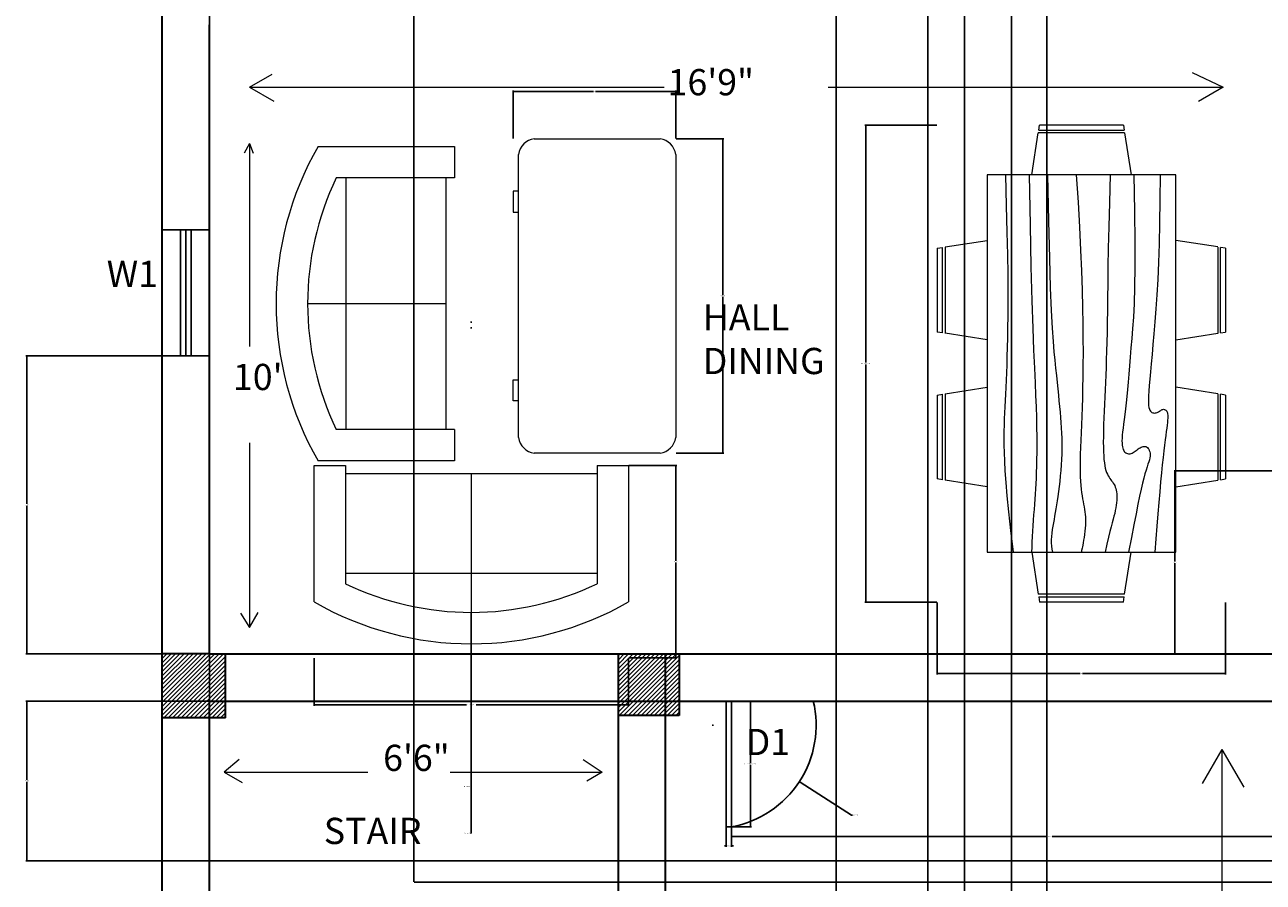
# Model space of a CAD drawing. Units: inches. Extents: x -4 to 429, y -457 to 84.
# Tile 2 of 4: x -4 to 232, y -295 to -131. Entities that reach past the tile are written whole.
import ezdxf

# ---------------------------------------------------------------- set-up
doc = ezdxf.new("R2010")
doc.units = ezdxf.units.IN
doc.header["$MEASUREMENT"] = 0
for name, color, linetype, lineweight in [('A-ANNO-DIMS', 2, 'Continuous', 18), ('A-ANNO-TEXT', 3, 'Continuous', 18), ('A-AREA-IDEN', 7, 'Continuous', 25), ('A-COLS', 7, 'Continuous', 35), ('A-COLS-PATT', 252, 'Continuous', 13), ('A-DOOR', 3, 'Continuous', 25), ('A-FURN', 8, 'Continuous', 18), ('A-GLAZ', 4, 'Continuous', 25), ('A-WALL', 7, 'Continuous', 35)]:
    doc.layers.add(name, color=color, linetype=linetype, lineweight=lineweight)
doc.styles.get("Standard").update_dxf_attribs({"font": 'arial.ttf'})
doc.dimstyles.get("Standard").update_dxf_attribs({"dimtxt": 0.18, "dimasz": 0.18, "dimexe": 0.18, "dimexo": 0.0625, "dimgap": 0.09, "dimtad": 0, "dimtih": 1, "dimtoh": 1, "dimdec": 4, "dimzin": 0, "dimdsep": 46, "dimtxsty": 'Standard', "dimcen": 0.09, "dimadec": 0, "dimazin": 0, "dimtfac": 1, "dimtdec": 4, "dimtofl": 0, "dimtmove": 0, "dimatfit": 3, "dimfxl": 1, "dimtolj": 1, "dimtzin": 0, "dimarcsym": 0})
pattern_1 = [(45, (-1330.13025, -719.5531), (-0.41542523, 0.41542523), [])]

# ---------------------------------------------------------------- blocks, each defined once
blk = doc.blocks.new('Dining Set - 36 x 72 in.')
for p, q in [((-22.2343, 26.00059), (-23.4847, 17.99762)), ((-22.2304, 26), (-5.7608, 26)), ((-22, 27.5), (-22.1562, 26.50042)), ((-5.8416, 26.5), (-22.1534, 26.5)), ((-22, 27.5), (-6, 27.5)), ((-5.8437, 26.49966), (-6, 27.5)), ((-4.5152, 17.99762), (-5.7655, 25.99926)), ((5.7657, 26.00059), (4.5153, 17.99762)), ((5.7696, 26), (22.2392, 26)), ((6, 27.5), (5.8438, 26.50042)), ((22.1584, 26.5), (5.8466, 26.5)), ((6, 27.5), (22, 27.5)), ((22.1563, 26.49966), (22, 27.5)), ((23.4848, 17.99762), (22.2345, 25.99926)), ((36, 18), (-36, 18)), ((-36, 18), (-36, -18)), ((36, -18), (36, 18)), ((-44.0006, 8.23428), (-35.9976, 9.48474)), ((44.0006, 8.23428), (35.9976, 9.48474)), ((-45.5, 8), (-44.5004, 8.15617)), ((-45.5, 8), (-45.5, -8)), ((-44.5, -8.15843), (-44.5, 8.15338)), ((-44, 8.23041), (-44, -8.23915)), ((44, 8.23041), (44, -8.23915)), ((44.5, -8.15843), (44.5, 8.15338)), ((45.5, 8), (44.5005, 8.15617)), ((45.5, 8), (45.5, -8)), ((-44.4997, -8.15631), (-45.5, -8)), ((-35.9976, -9.48476), (-43.9993, -8.2345)), ((35.9976, -9.48476), (43.9993, -8.2345)), ((44.4997, -8.15631), (45.5, -8)), ((-36, -18), (36, -18)), ((-22.2343, -26.0006), (-23.4847, -17.99762)), ((-4.5152, -17.99762), (-5.7655, -25.99928)), ((5.7657, -26.0006), (4.5153, -17.99762)), ((23.4848, -17.99762), (22.2345, -25.99928)), ((-22.2304, -26), (-5.7608, -26)), ((-22, -27.5), (-22.1562, -26.50044)), ((-5.8416, -26.5), (-22.1534, -26.5)), ((-22, -27.5), (-6, -27.5)), ((-5.8437, -26.49967), (-6, -27.5)), ((5.7696, -26), (22.2392, -26)), ((6, -27.5), (5.8438, -26.50044)), ((22.1584, -26.5), (5.8466, -26.5)), ((6, -27.5), (22, -27.5)), ((22.1563, -26.49967), (22, -27.5))]:
    blk.add_line(p, q)
for points in [[(-36, 15), (-31.1772, 14.97754), (-26.8079, 14.91406), (-22.8538, 14.81543), (-19.276, 14.6875), (-16.0362, 14.53613), (-13.0957, 14.36718), (-10.4159, 14.18652), (-7.9583, 14), (-5.6904, 13.81315), (-3.6035, 13.63021), (-1.6954, 13.45508), (0.0365, 13.29166), (1.5945, 13.14388), (2.9811, 13.01562), (4.1988, 12.9108), (5.25, 12.83333), (6.1393, 12.78613), (6.8802, 12.76823), (7.4883, 12.77767), (7.9792, 12.8125), (8.3685, 12.87077), (8.6719, 12.95052), (8.9049, 13.0498), (9.0833, 13.16666), (9.2205, 13.29899), (9.3216, 13.44401), (9.3895, 13.59879), (9.4271, 13.76041), (9.4373, 13.92594), (9.4232, 14.09245), (9.3875, 14.257), (9.3333, 14.41666), (9.2638, 14.56917), (9.1836, 14.71484), (9.0975, 14.85465), (9.0104, 14.98958), (8.9272, 15.1206), (8.8529, 15.2487), (8.7922, 15.37483), (8.75, 15.5), (8.7305, 15.62467), (8.7344, 15.74739), (8.7617, 15.86621), (8.8125, 15.97916), (8.8867, 16.08431), (8.9844, 16.17968), (9.1055, 16.26334), (9.25, 16.33333), (9.4189, 16.38802), (9.6172, 16.42708), (9.8506, 16.45052), (10.125, 16.45833), (10.4463, 16.45052), (10.8203, 16.42708), (11.2529, 16.38802), (11.75, 16.33333), (12.3184, 16.26318), (12.9694, 16.17838), (13.7151, 16.07991), (14.5677, 15.96875), (15.5395, 15.84586), (16.6426, 15.71224), (17.8893, 15.56884), (19.2917, 15.41666), (20.859, 15.25667), (22.5879, 15.08984), (24.4721, 14.91715), (26.5052, 14.73958), (28.6809, 14.5581), (30.9929, 14.3737), (33.4347, 14.18733), (36, 14)], [(-36, 10), (-28.9766, 10.14274), (-23.1725, 10.20442), (-18.4241, 10.19775), (-14.5677, 10.13541), (-11.4399, 10.03011), (-8.877, 9.89453), (-6.7154, 9.74137), (-4.7917, 9.58333), (-2.9698, 9.43082), (-1.2246, 9.28515), (0.4415, 9.14534), (2.026, 9.01041), (3.5266, 8.87939), (4.9408, 8.7513), (6.266, 8.62516), (7.5, 8.5), (8.6411, 8.37549), (9.6914, 8.2539), (10.6538, 8.13818), (11.5312, 8.03125), (12.3267, 7.93603), (13.043, 7.85547), (13.6831, 7.79248), (14.25, 7.75), (14.7471, 7.7303), (15.1797, 7.73307), (15.5537, 7.75732), (15.875, 7.80208), (16.1494, 7.86637), (16.3828, 7.94922), (16.5811, 8.04964), (16.75, 8.16666), (16.8944, 8.29915), (17.0143, 8.44531), (17.1089, 8.60319), (17.1771, 8.77083), (17.218, 8.94629), (17.2305, 9.1276), (17.2137, 9.31282), (17.1667, 9.5), (17.0895, 9.6875), (16.987, 9.875), (16.8649, 10.0625), (16.7292, 10.25), (16.5856, 10.4375), (16.4401, 10.625), (16.2985, 10.8125), (16.1667, 11), (16.05, 11.18733), (15.9518, 11.3737), (15.8752, 11.5581), (15.8229, 11.73958), (15.798, 11.91715), (15.8034, 12.08984), (15.842, 12.25667), (15.9167, 12.41666), (16.0295, 12.56836), (16.1784, 12.70833), (16.3605, 12.83268), (16.5729, 12.9375), (16.8127, 13.01888), (17.0768, 13.07291), (17.3625, 13.0957), (17.6667, 13.08333), (17.9894, 13.03312), (18.3418, 12.94726), (18.7382, 12.82918), (19.1927, 12.68229), (19.7195, 12.51001), (20.3327, 12.31575), (21.0465, 12.10294), (21.875, 11.875), (22.8357, 11.63354), (23.959, 11.37304), (25.2786, 11.08618), (26.8282, 10.76562), (28.6414, 10.40405), (30.752, 9.99414), (33.1936, 9.52856), (36, 9)], [(-36, 5.5), (-30.7157, 5.3348), (-26.069, 5.20963), (-21.9946, 5.11767), (-18.4271, 5.05208), (-15.3009, 5.00602), (-12.5508, 4.97265), (-10.1112, 4.94515), (-7.9167, 4.91666), (-5.909, 4.88167), (-4.0586, 4.83984), (-2.3429, 4.79215), (-0.7396, 4.73958), (0.7739, 4.6831), (2.22, 4.6237), (3.6213, 4.56233), (5, 4.5), (6.373, 4.43782), (7.7344, 4.3776), (9.0723, 4.32129), (10.375, 4.27083), (11.6309, 4.22819), (12.8281, 4.19531), (13.9551, 4.17415), (15, 4.16666), (15.954, 4.17448), (16.819, 4.19791), (17.6001, 4.23698), (18.3021, 4.29166), (18.9299, 4.36198), (19.4883, 4.44791), (19.9823, 4.54948), (20.4167, 4.66666), (20.7969, 4.79899), (21.1302, 4.94401), (21.4245, 5.09879), (21.6875, 5.26041), (21.9271, 5.42594), (22.1511, 5.59245), (22.3672, 5.757), (22.5834, 5.91666), (22.8065, 6.06868), (23.0404, 6.21093), (23.2879, 6.34147), (23.5521, 6.45833), (23.8358, 6.55957), (24.142, 6.64323), (24.4735, 6.70735), (24.8334, 6.75), (25.2235, 6.76969), (25.642, 6.76692), (26.0858, 6.74267), (26.5521, 6.69791), (27.0379, 6.63362), (27.5404, 6.55078), (28.0565, 6.45036), (28.5834, 6.33333), (29.1242, 6.19987), (29.7071, 6.04687), (30.3661, 5.87044), (31.1354, 5.66666), (32.0493, 5.43164), (33.142, 5.16146), (34.4475, 4.85221), (36, 4.5)], [(-36, -1), (-30.7915, -0.6591), (-26.0195, -0.38216), (-21.6519, -0.16284), (-17.6563, 0.00521), (-14.0005, 0.12833), (-10.6523, 0.21289), (-7.5796, 0.26522), (-4.75, 0.29166), (-2.134, 0.29793), (0.2878, 0.28711), (2.5317, 0.26163), (4.6146, 0.22396), (6.5529, 0.17651), (8.3633, 0.12174), (10.0623, 0.06209), (11.6667, 0), (13.1899, -0.06201), (14.6341, -0.1211), (15.9982, -0.17432), (17.2813, -0.21875), (18.4823, -0.25147), (19.6003, -0.26953), (20.6343, -0.27002), (21.5834, -0.25), (22.4481, -0.20768), (23.2357, -0.14584), (23.9549, -0.06836), (24.6146, 0.02083), (25.2235, 0.11784), (25.7904, 0.21875), (26.3241, 0.31966), (26.8334, 0.41666), (27.3265, 0.50618), (27.8099, 0.58593), (28.2894, 0.65397), (28.7709, 0.70833), (29.2601, 0.74707), (29.763, 0.76823), (30.2855, 0.76985), (30.8334, 0.75), (31.4088, 0.70784), (31.9994, 0.64713), (32.589, 0.57275), (33.1615, 0.48958), (33.7008, 0.4025), (34.1908, 0.3164), (34.6153, 0.23616), (34.9584, 0.16666), (35.2099, 0.11165), (35.3848, 0.07031), (35.504, 0.04069), (35.5886, 0.02083), (35.6594, 0.00879), (35.7377, 0.0026), (35.8442, 0.00032), (36, 0)], [(-36, -6.5), (-27.1843, -6.31267), (-20.084, -6.1263), (-14.469, -5.9419), (-10.1094, -5.76042), (-6.7752, -5.58285), (-4.2363, -5.41016), (-2.2629, -5.24333), (-0.625, -5.08334), (0.8708, -4.93099), (2.2715, -4.78646), (3.5872, -4.64974), (4.8281, -4.52084), (6.0046, -4.39974), (7.127, -4.28646), (8.2053, -4.18099), (9.25, -4.08334), (10.2705, -3.99382), (11.2734, -3.91407), (12.2647, -3.84603), (13.25, -3.79167), (14.2354, -3.75293), (15.2266, -3.73177), (16.2295, -3.73015), (17.25, -3.75), (18.2912, -3.79248), (19.3451, -3.85547), (20.4009, -3.93604), (21.4479, -4.03125), (22.4754, -4.13819), (23.4727, -4.25391), (24.4289, -4.37549), (25.3334, -4.5), (26.1785, -4.62492), (26.9694, -4.74935), (27.7145, -4.87281), (28.4219, -4.99479), (29.1, -5.11483), (29.7572, -5.23242), (30.4016, -5.34709), (31.0417, -5.45834), (31.6837, -5.56437), (32.3262, -5.65821), (32.9658, -5.73153), (33.599, -5.77604), (34.2224, -5.78345), (34.8327, -5.74545), (35.4264, -5.65373), (36, -5.5)], [(-36, -10), (-26.4022, -9.81299), (-18.4675, -9.62891), (-11.9839, -9.45069), (-6.7396, -9.28125), (-2.5226, -9.12354), (0.8789, -8.98047), (3.6769, -8.85498), (6.0833, -8.75), (8.2767, -8.66765), (10.3021, -8.60677), (12.1712, -8.56543), (13.8958, -8.54167), (15.4876, -8.53353), (16.9583, -8.53907), (18.3197, -8.55632), (19.5834, -8.58334), (20.7616, -8.61841), (21.8685, -8.66081), (22.9188, -8.71004), (23.9271, -8.76563), (24.9081, -8.82707), (25.8763, -8.89388), (26.8465, -8.96558), (27.8334, -9.04167), (28.8474, -9.12118), (29.8828, -9.20117), (30.93, -9.27824), (31.9792, -9.34896), (33.0205, -9.40991), (34.0443, -9.45768), (35.0407, -9.48885), (36, -9.5)], [(-36, -14.5), (-30.0881, -14.33513), (-25.0332, -14.21224), (-20.7312, -14.12647), (-17.0781, -14.07292), (-13.97, -14.04671), (-11.3027, -14.04297), (-8.9724, -14.05681), (-6.875, -14.08334), (-4.9224, -14.11833), (-3.0905, -14.16016), (-1.3709, -14.20785), (0.2448, -14.26042), (1.7647, -14.3169), (3.1973, -14.3763), (4.5507, -14.43767), (5.8333, -14.5), (7.0554, -14.5621), (8.235, -14.62175), (9.3922, -14.67652), (10.5469, -14.72396), (11.7192, -14.76164), (12.929, -14.78711), (14.1965, -14.79794), (15.5417, -14.79167), (16.9933, -14.76424), (18.6152, -14.70508), (20.4804, -14.60197), (22.6615, -14.44271), (25.2312, -14.21509), (28.2624, -13.9069), (31.8277, -13.50594), (36, -13)]]:
    blk.add_lwpolyline(points)
blk = doc.blocks.new('Sofa - Roundback Loveseat 5 ft.')
for p, q in [((0, -32.44198), (0, -5.99998)), ((-24, -33.99998), (-24, -11.46958)), ((24.00004, -33.99998), (24.00004, -11.46958)), ((-23.9998, -13.38178), (23.99986, -13.38178)), ((-24, -32.44198), (24.00004, -32.44198))]:
    blk.add_line(p, q)
for points in [[(-24, -33.99998), (-30, -33.99998), (-30, -7.99998)], [(30.00004, -7.99998), (30.00004, -33.99998), (24.00004, -33.99998)]]:
    blk.add_lwpolyline(points)
for centre, radius, start, end in [((0, -60.24998), 60.24998, 60.13715, 119.8628), ((0, -61.38438), 55.38444, 64.32083, 115.6792)]:
    blk.add_arc(centre, radius, start, end)
blk = doc.blocks.new('Desk - 30 x 60 in.')
for p, q in [((-26.999995, 0), (26.999995, 0)), ((-29.999995, -27), (-29.999995, -3)), ((29.999995, -3), (29.999995, -27)), ((26.999995, -30), (-26.999995, -30)), ((-20.000005, -30), (-20.000005, -31)), ((-16.000005, -31), (-16.000005, -30)), ((15.999995, -31), (15.999995, -30)), ((19.999995, -30), (19.999995, -31)), ((-20.000005, -31), (-16.000005, -31)), ((19.999995, -31), (15.999995, -31))]:
    blk.add_line(p, q)
for centre, start, end in [((-26.499995, -3.5), 98.1301, 171.8699), ((26.499995, -3.5), 8.130102, 81.8699), ((-26.499995, -26.5), 188.1301, 261.8699), ((26.499995, -26.5), 278.1301, 351.8699)]:
    blk.add_arc(centre, 3.535534, start, end)
blk = doc.blocks.new('WIN-24IN-9IN-WALL')
for p, q in [((0, 5.5), (24, 5.5)), ((0, 4.5), (24, 4.5)), ((0, 3.5), (24, 3.5))]:
    blk.add_line(p, q)
blk.add_lwpolyline([(0, 9), (24, 9), (24, 0), (0, 0)], close=True)
blk = doc.blocks.new('DOOR-LEAF-24IN')
for p, q in [((0, 0), (0, 24)), ((0, 24), (1, 24)), ((1, 24), (1, 0))]:
    blk.add_line(p, q)
blk = doc.blocks.new('*D14')
at = {"layer": 'A-ANNO-DIMS', "color": 0, "lineweight": -2, "transparency": 16777216}
for p, q in [((130.7, -260.34), (134.41, -260.34)), ((134.23, -260.52), (134.23, -272.16)), ((134.23, -284.16), (134.23, -272.52)), ((130.7, -284.34), (134.41, -284.34))]:
    blk.add_line(p, q, dxfattribs=at)
at = {"layer": 'A-ANNO-DIMS', "color": 0, "transparency": 16777216}
for points in [[(134.2, -260.52), (134.26, -260.52), (134.23, -260.34)], [(134.2, -284.16), (134.26, -284.16), (134.23, -284.34)]]:
    blk.add_solid(points, dxfattribs=at)
at = {"layer": 'Defpoints', "color": 0, "transparency": 16777216}
for p in [(130.63, -260.34), (130.63, -284.34), (134.23, -284.34)]:
    blk.add_point(p, dxfattribs=at)
at = {"layer": 'A-ANNO-DIMS', "color": 0, "transparency": 16777216, "insert": (134.23, -272.34), "char_height": 0.18, "attachment_point": 5}
blk.add_mtext('\\A1;DOOR LEAF 24 TYP.', dxfattribs=at)
blk = doc.blocks.new('*D15')
at = {"layer": 'A-ANNO-DIMS', "color": 0, "lineweight": -2, "transparency": 16777216}
for p, q in [((129.63, -284.4), (129.63, -288.12)), ((130.63, -284.4), (130.63, -288.12)), ((129.45, -287.94), (129.27, -287.94)), ((130.81, -287.94), (130.99, -287.94))]:
    blk.add_line(p, q, dxfattribs=at)
at = {"layer": 'A-ANNO-DIMS', "color": 0, "transparency": 16777216}
for points in [[(129.45, -287.91), (129.45, -287.97), (129.63, -287.94)], [(130.81, -287.91), (130.81, -287.97), (130.63, -287.94)]]:
    blk.add_solid(points, dxfattribs=at)
at = {"layer": 'Defpoints', "color": 0, "transparency": 16777216}
for p in [(129.63, -284.34), (130.63, -284.34), (129.63, -287.94)]:
    blk.add_point(p, dxfattribs=at)
at = {"layer": 'A-ANNO-DIMS', "color": 0, "transparency": 16777216, "insert": (130.13, -287.94), "char_height": 0.18, "attachment_point": 5}
blk.add_mtext('\\A1;1 TYP.', dxfattribs=at)
blk = doc.blocks.new('*D18')
at = {"layer": 'A-ANNO-DIMS', "color": 0, "lineweight": -2, "transparency": 16777216}
for p, q in [((51, -252.15), (51, -261.27)), ((111, -252.15), (111, -261.27)), ((51.18, -261.09), (80.1, -261.09)), ((110.82, -261.09), (81.91, -261.09))]:
    blk.add_line(p, q, dxfattribs=at)
at = {"layer": 'A-ANNO-DIMS', "color": 0, "transparency": 16777216}
for points in [[(51.18, -261.06), (51.18, -261.12), (51, -261.09)], [(110.82, -261.06), (110.82, -261.12), (111, -261.09)]]:
    blk.add_solid(points, dxfattribs=at)
at = {"layer": 'Defpoints', "color": 0, "transparency": 16777216}
for p in [(51, -252.09), (111, -252.09), (51, -261.09)]:
    blk.add_point(p, dxfattribs=at)
at = {"layer": 'A-ANNO-DIMS', "color": 0, "transparency": 16777216, "insert": (81, -261.09), "char_height": 0.18, "attachment_point": 5}
blk.add_mtext('\\A1;SOFA 60 TYP.', dxfattribs=at)
blk = doc.blocks.new('*D19')
at = {"layer": 'A-ANNO-DIMS', "color": 0, "lineweight": -2, "transparency": 16777216}
for p, q in [((111.06, -215.42), (120.18, -215.42)), ((120, -215.6), (120, -233.57)), ((120, -251.91), (120, -233.94)), ((111.06, -252.09), (120.18, -252.09))]:
    blk.add_line(p, q, dxfattribs=at)
at = {"layer": 'A-ANNO-DIMS', "color": 0, "transparency": 16777216}
for points in [[(119.97, -215.6), (120.03, -215.6), (120, -215.42)], [(119.97, -251.91), (120.03, -251.91), (120, -252.09)]]:
    blk.add_solid(points, dxfattribs=at)
at = {"layer": 'Defpoints', "color": 0, "transparency": 16777216}
for p in [(111, -215.42), (111, -252.09), (120, -252.09)]:
    blk.add_point(p, dxfattribs=at)
at = {"layer": 'A-ANNO-DIMS', "color": 0, "transparency": 16777216, "insert": (120, -233.76), "char_height": 0.18, "attachment_point": 5}
blk.add_mtext('\\A1;37 TYP.', dxfattribs=at)
blk = doc.blocks.new('*D24')
at = {"layer": 'A-ANNO-DIMS', "color": 0, "lineweight": -2, "transparency": 16777216}
for p, q in [((169.81, -150.46), (156.04, -150.46)), ((156.22, -150.64), (156.22, -195.78)), ((156.22, -241.28), (156.22, -196.15)), ((169.81, -241.46), (156.04, -241.46))]:
    blk.add_line(p, q, dxfattribs=at)
at = {"layer": 'A-ANNO-DIMS', "color": 0, "transparency": 16777216}
for points in [[(156.19, -150.64), (156.25, -150.64), (156.22, -150.46)], [(156.19, -241.28), (156.25, -241.28), (156.22, -241.46)]]:
    blk.add_solid(points, dxfattribs=at)
at = {"layer": 'Defpoints', "color": 0, "transparency": 16777216}
for p in [(169.87, -150.46), (156.22, -241.46), (169.87, -241.46)]:
    blk.add_point(p, dxfattribs=at)
at = {"layer": 'A-ANNO-DIMS', "color": 0, "transparency": 16777216, "insert": (156.22, -195.96), "char_height": 0.18, "attachment_point": 5}
blk.add_mtext('\\A1;DINING SET 91', dxfattribs=at)
blk = doc.blocks.new('*D25')
at = {"layer": 'A-ANNO-DIMS', "color": 0, "lineweight": -2, "transparency": 16777216}
for p, q in [((169.87, -241.53), (169.87, -255.29)), ((224.87, -241.53), (224.87, -255.29)), ((170.05, -255.11), (197.15, -255.11)), ((224.69, -255.11), (197.59, -255.11))]:
    blk.add_line(p, q, dxfattribs=at)
at = {"layer": 'A-ANNO-DIMS', "color": 0, "transparency": 16777216}
for points in [[(170.05, -255.08), (170.05, -255.14), (169.87, -255.11)], [(224.69, -255.08), (224.69, -255.14), (224.87, -255.11)]]:
    blk.add_solid(points, dxfattribs=at)
at = {"layer": 'Defpoints', "color": 0, "transparency": 16777216}
for p in [(169.87, -241.46), (224.87, -241.46), (224.87, -255.11)]:
    blk.add_point(p, dxfattribs=at)
at = {"layer": 'A-ANNO-DIMS', "color": 0, "transparency": 16777216, "insert": (197.37, -255.11), "char_height": 0.18, "attachment_point": 5}
blk.add_mtext('\\A1;55', dxfattribs=at)
blk = doc.blocks.new('*D26')
at = {"layer": 'A-ANNO-DIMS', "color": 0, "lineweight": -2, "transparency": 16777216}
for p, q in [((120.06, -153.07), (129.18, -153.07)), ((129, -153.25), (129, -182.89)), ((129, -212.89), (129, -183.25)), ((120.06, -213.07), (129.18, -213.07))]:
    blk.add_line(p, q, dxfattribs=at)
at = {"layer": 'A-ANNO-DIMS', "color": 0, "transparency": 16777216}
for points in [[(128.97, -153.25), (129.03, -153.25), (129, -153.07)], [(128.97, -212.89), (129.03, -212.89), (129, -213.07)]]:
    blk.add_solid(points, dxfattribs=at)
at = {"layer": 'Defpoints', "color": 0, "transparency": 16777216}
for p in [(120, -153.07), (120, -213.07), (129, -213.07)]:
    blk.add_point(p, dxfattribs=at)
at = {"layer": 'A-ANNO-DIMS', "color": 0, "transparency": 16777216, "insert": (129, -183.07), "char_height": 0.18, "attachment_point": 5}
blk.add_mtext('\\A1;DESK 60', dxfattribs=at)
blk = doc.blocks.new('*D27')
at = {"layer": 'A-ANNO-DIMS', "color": 0, "lineweight": -2, "transparency": 16777216}
for p, q in [((89, -153.01), (89, -143.89)), ((89.18, -144.07), (104.3, -144.07)), ((119.82, -144.07), (104.7, -144.07)), ((120, -153.01), (120, -143.89))]:
    blk.add_line(p, q, dxfattribs=at)
at = {"layer": 'A-ANNO-DIMS', "color": 0, "transparency": 16777216}
for points in [[(89.18, -144.04), (89.18, -144.1), (89, -144.07)], [(119.82, -144.04), (119.82, -144.1), (120, -144.07)]]:
    blk.add_solid(points, dxfattribs=at)
at = {"layer": 'Defpoints', "color": 0, "transparency": 16777216}
for p in [(120, -144.07), (89, -153.07), (120, -153.07)]:
    blk.add_point(p, dxfattribs=at)
at = {"layer": 'A-ANNO-DIMS', "color": 0, "transparency": 16777216, "insert": (104.5, -144.07), "char_height": 0.18, "attachment_point": 5}
blk.add_mtext('\\A1;31', dxfattribs=at)
blk = doc.blocks.new('*D32')
at = {"layer": 'A-ANNO-DIMS', "color": 0, "lineweight": -2, "transparency": 16777216}
for p, q in [((31.06, -294.84), (31.06, 84.09)), ((31.24, 83.91), (50.34, 83.91)), ((69.88, 83.91), (50.78, 83.91)), ((70.06, -294.84), (70.06, 84.09))]:
    blk.add_line(p, q, dxfattribs=at)
at = {"layer": 'A-ANNO-DIMS', "color": 0, "transparency": 16777216}
for points in [[(31.24, 83.94), (31.24, 83.88), (31.06, 83.91)], [(69.88, 83.94), (69.88, 83.88), (70.06, 83.91)]]:
    blk.add_solid(points, dxfattribs=at)
at = {"layer": 'Defpoints', "color": 0, "transparency": 16777216}
for p in [(70.06, 83.91), (31.06, -294.9), (70.06, -294.9)]:
    blk.add_point(p, dxfattribs=at)
at = {"layer": 'A-ANNO-DIMS', "color": 0, "transparency": 16777216, "insert": (50.56, 83.91), "char_height": 0.18, "attachment_point": 5}
blk.add_mtext('\\A1;39', dxfattribs=at)
blk = doc.blocks.new('*D33')
at = {"layer": 'A-ANNO-DIMS', "color": 0, "lineweight": -2, "transparency": 16777216}
for p, q in [((70.12, -294.9), (429.31, -294.9)), ((429.13, -295.08), (429.13, -299.22)), ((429.13, -303.72), (429.13, -299.59)), ((70.12, -303.9), (429.31, -303.9))]:
    blk.add_line(p, q, dxfattribs=at)
at = {"layer": 'A-ANNO-DIMS', "color": 0, "transparency": 16777216}
for points in [[(429.1, -295.08), (429.16, -295.08), (429.13, -294.9)], [(429.1, -303.72), (429.16, -303.72), (429.13, -303.9)]]:
    blk.add_solid(points, dxfattribs=at)
at = {"layer": 'Defpoints', "color": 0, "transparency": 16777216}
for p in [(70.06, -294.9), (70.06, -303.9), (429.13, -303.9)]:
    blk.add_point(p, dxfattribs=at)
at = {"layer": 'A-ANNO-DIMS', "color": 0, "transparency": 16777216, "insert": (429.13, -299.4), "char_height": 0.18, "attachment_point": 5}
blk.add_mtext('\\A1;9', dxfattribs=at)
blk = doc.blocks.new('*D35')
at = {"layer": 'A-ANNO-DIMS', "color": 0, "lineweight": -2, "transparency": 16777216}
for p, q in [((150.6, -85.07), (150.6, -457.42)), ((175.06, -85.07), (175.06, -457.42)), ((150.78, -457.24), (162.36, -457.24)), ((174.88, -457.24), (163.29, -457.24))]:
    blk.add_line(p, q, dxfattribs=at)
at = {"layer": 'A-ANNO-DIMS', "color": 0, "transparency": 16777216}
for points in [[(150.78, -457.21), (150.78, -457.27), (150.6, -457.24)], [(174.88, -457.21), (174.88, -457.27), (175.06, -457.24)]]:
    blk.add_solid(points, dxfattribs=at)
at = {"layer": 'Defpoints', "color": 0, "transparency": 16777216}
for p in [(150.6, -85.01), (175.06, -85.01), (175.06, -457.24)]:
    blk.add_point(p, dxfattribs=at)
at = {"layer": 'A-ANNO-DIMS', "color": 0, "transparency": 16777216, "insert": (162.83, -457.24), "char_height": 0.18, "attachment_point": 5}
blk.add_mtext('\\A1;24.457', dxfattribs=at)
blk = doc.blocks.new('*D37')
at = {"layer": 'A-ANNO-DIMS', "color": 0, "lineweight": -2, "transparency": 16777216}
for p, q in [((240.99, -216.42), (215.03, -216.42)), ((215.21, -216.6), (215.21, -233.7)), ((215.21, -251.16), (215.21, -234.06)), ((240.99, -251.34), (215.03, -251.34))]:
    blk.add_line(p, q, dxfattribs=at)
at = {"layer": 'A-ANNO-DIMS', "color": 0, "transparency": 16777216}
for points in [[(215.18, -216.6), (215.24, -216.6), (215.21, -216.42)], [(215.18, -251.16), (215.24, -251.16), (215.21, -251.34)]]:
    blk.add_solid(points, dxfattribs=at)
at = {"layer": 'Defpoints', "color": 0, "transparency": 16777216}
for p in [(215.21, -216.42), (241.06, -216.42), (241.06, -251.34)]:
    blk.add_point(p, dxfattribs=at)
at = {"layer": 'A-ANNO-DIMS', "color": 0, "transparency": 16777216, "insert": (215.21, -233.88), "char_height": 0.18, "attachment_point": 5}
blk.add_mtext('\\A1;34.92', dxfattribs=at)
blk = doc.blocks.new('*D41')
at = {"layer": 'A-ANNO-DIMS', "color": 0, "lineweight": -2, "transparency": 16777216}
for p, q in [((324.99, -260.34), (-3.97, -260.34)), ((-3.79, -260.52), (-3.79, -275.4)), ((-3.79, -290.65), (-3.79, -275.76)), ((324.99, -290.83), (-3.97, -290.83))]:
    blk.add_line(p, q, dxfattribs=at)
at = {"layer": 'A-ANNO-DIMS', "color": 0, "transparency": 16777216}
for points in [[(-3.82, -260.52), (-3.76, -260.52), (-3.79, -260.34)], [(-3.82, -290.65), (-3.76, -290.65), (-3.79, -290.83)]]:
    blk.add_solid(points, dxfattribs=at)
at = {"layer": 'Defpoints', "color": 0, "transparency": 16777216}
for p in [(325.06, -260.34), (-3.79, -290.83), (325.06, -290.83)]:
    blk.add_point(p, dxfattribs=at)
at = {"layer": 'A-ANNO-DIMS', "color": 0, "transparency": 16777216, "insert": (-3.79, -275.58), "char_height": 0.18, "attachment_point": 5}
blk.add_mtext('\\A1;30.486', dxfattribs=at)
blk = doc.blocks.new('*D43')
at = {"layer": 'A-ANNO-DIMS', "color": 0, "lineweight": -2, "transparency": 16777216}
for p, q in [((21.99, -194.47), (-3.97, -194.47)), ((-3.79, -194.65), (-3.79, -222.72)), ((-3.79, -251.16), (-3.79, -223.09)), ((21.99, -251.34), (-3.97, -251.34))]:
    blk.add_line(p, q, dxfattribs=at)
at = {"layer": 'A-ANNO-DIMS', "color": 0, "transparency": 16777216}
for points in [[(-3.82, -194.65), (-3.76, -194.65), (-3.79, -194.47)], [(-3.82, -251.16), (-3.76, -251.16), (-3.79, -251.34)]]:
    blk.add_solid(points, dxfattribs=at)
at = {"layer": 'Defpoints', "color": 0, "transparency": 16777216}
for p in [(22.06, -194.47), (-3.79, -251.34), (22.06, -251.34)]:
    blk.add_point(p, dxfattribs=at)
at = {"layer": 'A-ANNO-DIMS', "color": 0, "transparency": 16777216, "insert": (-3.79, -222.9), "char_height": 0.18, "attachment_point": 5}
blk.add_mtext('\\A1;56.87', dxfattribs=at)
blk = doc.blocks.new('*D48')
at = {"layer": 'A-ANNO-DIMS', "color": 0, "lineweight": -2, "transparency": 16777216}
for p, q in [((130.63, -260.4), (130.63, -286.37)), ((252.06, -260.4), (252.06, -286.37)), ((130.81, -286.19), (190.89, -286.19)), ((251.88, -286.19), (191.8, -286.19))]:
    blk.add_line(p, q, dxfattribs=at)
at = {"layer": 'A-ANNO-DIMS', "color": 0, "transparency": 16777216}
for points in [[(130.81, -286.16), (130.81, -286.22), (130.63, -286.19)], [(251.88, -286.16), (251.88, -286.22), (252.06, -286.19)]]:
    blk.add_solid(points, dxfattribs=at)
at = {"layer": 'Defpoints', "color": 0, "transparency": 16777216}
for p in [(130.63, -260.34), (252.06, -260.34), (130.63, -286.19)]:
    blk.add_point(p, dxfattribs=at)
at = {"layer": 'A-ANNO-DIMS', "color": 0, "transparency": 16777216, "insert": (191.35, -286.19), "char_height": 0.18, "attachment_point": 5}
blk.add_mtext('\\A1;121.42', dxfattribs=at)
blk = doc.blocks.new('*D51')
at = {"layer": 'A-ANNO-DIMS', "color": 0, "lineweight": -2, "transparency": 16777216}
for p, q in [((175.06, -118.1), (175.06, -457.42)), ((168.05, -122.4), (168.05, -457.42)), ((168.23, -457.24), (171.16, -457.24)), ((174.88, -457.24), (171.95, -457.24))]:
    blk.add_line(p, q, dxfattribs=at)
at = {"layer": 'A-ANNO-DIMS', "color": 0, "transparency": 16777216}
for points in [[(168.23, -457.21), (168.23, -457.27), (168.05, -457.24)], [(174.88, -457.21), (174.88, -457.27), (175.06, -457.24)]]:
    blk.add_solid(points, dxfattribs=at)
at = {"layer": 'Defpoints', "color": 0, "transparency": 16777216}
for p in [(175.06, -118.04), (168.05, -122.34), (175.06, -457.24)]:
    blk.add_point(p, dxfattribs=at)
at = {"layer": 'A-ANNO-DIMS', "color": 0, "transparency": 16777216, "insert": (171.56, -457.24), "char_height": 0.18, "attachment_point": 5}
blk.add_mtext('\\A1;7.002', dxfattribs=at)
blk = doc.blocks.new('*D52')
at = {"layer": 'A-ANNO-DIMS', "color": 0, "lineweight": -2, "transparency": 16777216}
for p, q in [((184.06, -118.1), (184.06, -457.42)), ((190.77, -122.4), (190.77, -457.42)), ((184.24, -457.24), (187.02, -457.24)), ((190.59, -457.24), (187.81, -457.24))]:
    blk.add_line(p, q, dxfattribs=at)
at = {"layer": 'A-ANNO-DIMS', "color": 0, "transparency": 16777216}
for points in [[(184.24, -457.21), (184.24, -457.27), (184.06, -457.24)], [(190.59, -457.21), (190.59, -457.27), (190.77, -457.24)]]:
    blk.add_solid(points, dxfattribs=at)
at = {"layer": 'Defpoints', "color": 0, "transparency": 16777216}
for p in [(184.06, -118.04), (190.77, -122.34), (190.77, -457.24)]:
    blk.add_point(p, dxfattribs=at)
at = {"layer": 'A-ANNO-DIMS', "color": 0, "transparency": 16777216, "insert": (187.41, -457.24), "char_height": 0.18, "attachment_point": 5}
blk.add_mtext('\\A1;6.714', dxfattribs=at)
blk = doc.blocks.new('*D59')
at = {"layer": 'A-ANNO-DIMS', "color": 0, "lineweight": -2, "transparency": 16777216}
for p, q in [((126.98, -264.97), (127.16, -264.97)), ((127.07, -265.06), (127.07, -264.88)), ((153.5, -282.13), (143.74, -275.79)), ((153.68, -282.13), (153.5, -282.13))]:
    blk.add_line(p, q, dxfattribs=at)
at = {"layer": 'A-ANNO-DIMS', "color": 0, "transparency": 16777216}
blk.add_solid([(143.76, -275.77), (143.72, -275.82), (143.59, -275.69)], dxfattribs=at)
at = {"layer": 'Defpoints', "color": 0, "transparency": 16777216}
for p in [(127.07, -264.97), (143.59, -275.69)]:
    blk.add_point(p, dxfattribs=at)
at = {"layer": 'A-ANNO-DIMS', "color": 0, "transparency": 16777216, "insert": (154.23, -282.13), "char_height": 0.18, "attachment_point": 5}
blk.add_mtext('\\A1;R19.695', dxfattribs=at)
blk = doc.blocks.new('*D60')
at = {"layer": 'A-ANNO-DIMS', "color": 0, "lineweight": -2, "transparency": 16777216}
for p, q in [((80.91, -189.17), (81.09, -189.17)), ((81, -189.26), (81, -189.08)), ((81, -285.57), (81, -249.6)), ((80.82, -285.57), (81, -285.57))]:
    blk.add_line(p, q, dxfattribs=at)
at = {"layer": 'A-ANNO-DIMS', "color": 0, "transparency": 16777216}
blk.add_solid([(80.97, -249.6), (81.03, -249.6), (81, -249.42)], dxfattribs=at)
at = {"layer": 'Defpoints', "color": 0, "transparency": 16777216}
for p in [(81, -189.17), (81, -249.42)]:
    blk.add_point(p, dxfattribs=at)
at = {"layer": 'A-ANNO-DIMS', "color": 0, "transparency": 16777216, "insert": (80.15, -285.57), "char_height": 0.18, "attachment_point": 5}
blk.add_mtext('\\A1;2X R60.25', dxfattribs=at)
blk = doc.blocks.new('*D61')
at = {"layer": 'A-ANNO-DIMS', "color": 0, "lineweight": -2, "transparency": 16777216}
for p, q in [((80.91, -188.04), (81.09, -188.04)), ((81, -188.13), (81, -187.95)), ((81, -276.65), (81, -243.6)), ((80.82, -276.65), (81, -276.65))]:
    blk.add_line(p, q, dxfattribs=at)
at = {"layer": 'A-ANNO-DIMS', "color": 0, "transparency": 16777216}
blk.add_solid([(80.97, -243.6), (81.03, -243.6), (81, -243.42)], dxfattribs=at)
at = {"layer": 'Defpoints', "color": 0, "transparency": 16777216}
for p in [(81, -188.04), (81, -243.42)]:
    blk.add_point(p, dxfattribs=at)
at = {"layer": 'A-ANNO-DIMS', "color": 0, "transparency": 16777216, "insert": (80.15, -276.65), "char_height": 0.18, "attachment_point": 5}
blk.add_mtext('\\A1;2X R55.38', dxfattribs=at)

msp = doc.modelspace()

# ---------------------------------------------------------------- hatches: boundary and pattern name
at = {"layer": 'A-COLS-PATT'}
h = msp.add_hatch(dxfattribs=at)
h.set_pattern_fill('ANSI31', color=256, scale=4.7)
h.set_pattern_definition(pattern_1)
h.paths.add_polyline_path([(334.0572, -251.3399), (325.0572, -251.3399), (319.9964, -251.3399), (319.9964, -260.3399), (325.0572, -260.3399), (325.0572, -263.4636), (334.0572, -263.4636)])
h.paths.add_polyline_path([(325.0572, -260.3399), (319.9964, -260.3399), (319.9964, -263.4636), (325.0572, -263.4636)], flags=17)
h.paths.add_polyline_path([(34.0899, -251.3399), (31.0572, -251.3399), (22.0572, -251.3399), (22.0572, -263.5568), (31.0572, -263.5568), (31.0572, -260.3399), (34.0899, -260.3399)])
h.paths.add_polyline_path([(34.0899, -260.3399), (31.0572, -260.3399), (31.0572, -263.5568), (34.0899, -263.5568)], flags=17)
h = msp.add_hatch(dxfattribs=at)
h.set_pattern_fill('ANSI31', color=256, scale=4.7)
h.set_pattern_definition(pattern_1)
h.paths.add_polyline_path([(118.0572, -251.3399), (109.0572, -251.3399), (109.0572, -260.3399), (118.0572, -260.3399)])
h.paths.add_polyline_path([(120.644, -260.3399), (118.0572, -260.3399), (118.0572, -263.095), (120.644, -263.095)])
h.paths.add_polyline_path([(118.0572, -260.3399), (109.0572, -260.3399), (109.0572, -263.095), (118.0572, -263.095)])
h.paths.add_polyline_path([(120.644, -251.3399), (118.0572, -251.3399), (118.0572, -260.3399), (120.644, -260.3399)])

# ---------------------------------------------------------------- linework, layer by layer
at = {"layer": 'A-ANNO-DIMS'}
for p, q in [((38.7181, -143.2364), (43.0487, -140.7361)), ((218.4656, -140.4219), (224.4316, -143.2364)), ((38.7181, -143.2364), (117.7941, -143.2364)), ((38.7181, -143.2364), (43.3477, -145.9093)), ((149.0432, -143.2364), (224.4316, -143.2364)), ((224.4316, -143.2364), (219.6865, -145.9759)), ((38.7181, -154.0146), (37.6723, -155.8259)), ((38.7181, -154.0146), (38.7181, -192.7253)), ((38.7181, -154.0146), (39.3909, -155.8205)), ((38.7181, -211.1032), (38.7181, -246.2948)), ((36.9802, -243.6005), (38.7181, -246.2948)), ((38.7181, -246.2948), (40.3576, -243.455)), ((36.7526, -271.4623), (33.8944, -273.9035)), ((102.3193, -271.4644), (105.9894, -273.9035)), ((224.1656, -269.5865), (220.4053, -276.0995)), ((224.1656, -269.5865), (224.1656, -327.7164)), ((224.1656, -269.5865), (228.3289, -276.7976)), ((33.8944, -273.9035), (61.2806, -273.9035)), ((33.8944, -273.9035), (37.3225, -275.8828)), ((76.9534, -273.9035), (105.9894, -273.9035)), ((105.9894, -273.9035), (103.0555, -275.5974))]:
    msp.add_line(p, q, dxfattribs=at)
at = {"layer": 'A-COLS'}
for p, q in [((31.0572, -251.3399), (22.0572, -251.3399)), ((34.0899, -263.5568), (34.0899, -251.3399)), ((120.644, -251.3399), (120.644, -263.095)), ((34.0899, -263.5568), (22.0572, -263.5568)), ((120.644, -263.095), (109.0572, -263.095))]:
    msp.add_line(p, q, dxfattribs=at)
at = {"layer": 'A-DOOR'}
msp.add_arc((127.0685, -264.9701), 19.6952, 280.429569, 13.597072, dxfattribs=at)
at = {"layer": 'A-WALL'}
for p, q in [((31.0572, -251.3399), (31.0572, -131.3399)), ((31.0572, -251.3399), (325.0572, -251.3399)), ((109.0572, -422.3399), (109.0572, -251.3399)), ((118.0572, -422.3399), (118.0572, -251.3399)), ((31.0572, -422.3399), (31.0572, -260.3399)), ((31.0572, -260.3399), (325.0572, -260.3399))]:
    msp.add_line(p, q, dxfattribs=at)
msp.add_lwpolyline([(22.0572, 18.6601), (334.0572, 18.6601), (334.0572, -431.3399), (22.0572, -431.3399)], close=True, dxfattribs=at)

# ---------------------------------------------------------------- block references
at = {"layer": 'A-DOOR', "rotation": 180}
msp.add_blockref('DOOR-LEAF-24IN', (130.634, -260.3398), dxfattribs=at)
at = {"layer": 'A-FURN'}
for name, p, rotation in [('Dining Set - 36 x 72 in.', (197.374, -195.9644), 270), ('Desk - 30 x 60 in.', (120.0023, -183.0695), 270), ('Sofa - Roundback Loveseat 5 ft.', (43.7804, -184.5509), 89.99999999999999), ('Sofa - Roundback Loveseat 5 ft.', (81.0023, -249.4236), 180)]:
    msp.add_blockref(name, p, dxfattribs=dict(at, rotation=rotation))
at = {"layer": 'A-GLAZ', "extrusion": (0, 0, -1), "zscale": -1, "rotation": 270}
msp.add_blockref('WIN-24IN-9IN-WALL', (-31.0573, -170.4699), dxfattribs=at)

# ---------------------------------------------------------------- texts
at = {"layer": 'A-ANNO-DIMS', "char_height": 5, "attachment_point": 1}
for s, width, insert in [('16\'9"', 34.945791, (118.4328, -139.795)), ("10'", 7.799597, (35.5369, -196.0241)), ('6\'6"', 11.579515, (64.1777, -268.6808))]:
    msp.add_mtext_dynamic_manual_height_columns(s, width=width, gutter_width=25, heights=[0], dxfattribs=dict(at, insert=insert))
at = {"layer": 'A-ANNO-TEXT', "char_height": 5, "attachment_point": 1}
for s, width, insert in [('W1', 7.590927, (11.4683, -176.3531)), ('D1', 8.348311, (133.3314, -265.6506))]:
    msp.add_mtext_dynamic_manual_height_columns(s, width=width, gutter_width=25, heights=[0], dxfattribs=dict(at, insert=insert))
at = {"layer": 'A-AREA-IDEN', "char_height": 5, "attachment_point": 1}
for s, width, insert in [('HALL\\PDINING', 18.300299, (125.1469, -184.6436)), ('STAIR', 25.184408, (52.8634, -282.6139))]:
    msp.add_mtext_dynamic_manual_height_columns(s, width=width, gutter_width=25, heights=[0], dxfattribs=dict(at, insert=insert))

# ---------------------------------------------------------------- dimensions: what is measured, and where the dimension line sits
at = {"layer": 'A-ANNO-DIMS'}
for base, p1, p2, override, picture, middle in [((70.0572, 83.9133), (31.0572, -294.9035), (70.0572, -294.9035), {"dimdec": 0, "dimlfac": 1, "dimrnd": 0, "dimzin": 0, "dimdsep": 46, "dimlunit": 2}, '*D32', (50.5572, 83.9133)), ((175.0572, -457.2361), (150.6, -85.0072), (175.0572, -85.0072), {"dimdec": 3, "dimlfac": 1, "dimrnd": 0, "dimzin": 0, "dimdsep": 46, "dimlunit": 2}, '*D35', (162.8286, -457.2361)), ((175.0572, -457.2361), (168.0549, -122.3399), (175.0572, -118.0379), {"dimdec": 3, "dimlfac": 1, "dimrnd": 0, "dimzin": 0, "dimdsep": 46, "dimlunit": 2}, '*D51', (171.5561, -457.2361)), ((190.7712, -457.2361), (184.0572, -118.0379), (190.7712, -122.3399), {"dimdec": 3, "dimlfac": 1, "dimrnd": 0, "dimzin": 0, "dimdsep": 46, "dimlunit": 2}, '*D52', (187.4142, -457.2361)), ((120.0023, -144.0695), (89.0023, -153.0695), (120.0023, -153.0695), {"dimdec": 0, "dimlfac": 1, "dimrnd": 0, "dimzin": 0, "dimdsep": 46, "dimlunit": 2}, '*D27', (104.5023, -144.0695)), ((224.874, -255.1144), (169.874, -241.4644), (224.874, -241.4644), {"dimdec": 0, "dimlfac": 1, "dimrnd": 0, "dimzin": 0, "dimdsep": 46, "dimlunit": 2}, '*D25', (197.374, -255.1144))]:
    dim = msp.add_linear_dim(base=base, p1=p1, p2=p2, dimstyle='Standard', override=override, dxfattribs=at)
    dim.commit()
    dim.dimension.update_dxf_attribs({"geometry": picture, "text_midpoint": middle})
for base, p1, p2, angle, text, picture, middle in [((156.224, -241.4644), (169.874, -150.4644), (169.874, -241.4644), 270, 'DINING SET <>', '*D24', (156.224, -195.9644)), ((129.0023, -213.0695), (120.0023, -153.0695), (120.0023, -213.0695), 270, 'DESK <>', '*D26', (129.0023, -183.0695)), ((120.0024, -252.0903), (111.0023, -215.4236), (111.0023, -252.0903), 270, '<> TYP.', '*D19', (120.0024, -233.7569)), ((51.0023, -261.0903), (111.0023, -252.0903), (51.0023, -252.0903), 180, 'SOFA <> TYP.', '*D18', (81.0023, -261.0903)), ((134.2339, -284.3399), (130.6339, -260.3399), (130.6339, -284.3399), 270, 'DOOR LEAF <> TYP.', '*D14', (134.2339, -272.3399)), ((129.6339, -287.9399), (130.6339, -284.3399), (129.6339, -284.3399), 180, '<> TYP.', '*D15', (130.1339, -287.9399))]:
    dim = msp.add_linear_dim(base=base, p1=p1, p2=p2, angle=angle, text=text, dimstyle='Standard', override={"dimdec": 0, "dimlfac": 1, "dimrnd": 0, "dimzin": 0, "dimdsep": 46, "dimlunit": 2}, dxfattribs=at)
    dim.commit()
    dim.dimension.update_dxf_attribs({"geometry": picture, "text_midpoint": middle})
for center, mpoint, picture, middle in [((81.0023, -188.0392), (81.002, -243.4236), '*D61', (80.1469, -276.6543)), ((81.0023, -189.1736), (81.002, -249.4236), '*D60', (80.1464, -285.5736))]:
    dim = msp.add_radius_dim(center=center, mpoint=mpoint, text='2X <>', dimstyle='Standard', override={"dimdec": 2, "dimlfac": 1, "dimrnd": 0, "dimzin": 0, "dimdsep": 46, "dimlunit": 2}, dxfattribs=at)
    dim.commit()
    dim.dimension.update_dxf_attribs({"geometry": picture, "text_midpoint": middle, "dimtype": 164})
for base, p1, p2, angle, override, picture, middle in [((-3.7928, -251.3399), (22.0572, -194.4698), (22.0572, -251.3399), 90, {"dimdec": 2, "dimlfac": 1, "dimrnd": 0, "dimzin": 0, "dimdsep": 46, "dimlunit": 2}, '*D43', (-3.7928, -222.9048)), ((215.2072, -216.4188), (241.0572, -251.3399), (241.0572, -216.4188), 90, {"dimdec": 2, "dimlfac": 1, "dimrnd": 0, "dimzin": 0, "dimdsep": 46, "dimlunit": 2}, '*D37', (215.2072, -233.8794)), ((-3.7928, -290.8261), (325.0572, -260.3399), (325.0572, -290.8261), 90, {"dimdec": 3, "dimlfac": 1, "dimrnd": 0, "dimzin": 0, "dimdsep": 46, "dimlunit": 2}, '*D41', (-3.7928, -275.583)), ((130.6339, -286.1899), (252.0572, -260.3399), (130.6339, -260.3399), 180, {"dimdec": 2, "dimlfac": 1, "dimrnd": 0, "dimzin": 0, "dimdsep": 46, "dimlunit": 2}, '*D48', (191.3455, -286.1899)), ((429.1331, -303.9035), (70.0572, -294.9035), (70.0572, -303.9035), 90, {"dimdec": 0, "dimlfac": 1, "dimrnd": 0, "dimzin": 0, "dimdsep": 46, "dimlunit": 2}, '*D33', (429.1331, -299.4035))]:
    dim = msp.add_linear_dim(base=base, p1=p1, p2=p2, angle=angle, dimstyle='Standard', override=override, dxfattribs=at)
    dim.commit()
    dim.dimension.update_dxf_attribs({"geometry": picture, "text_midpoint": middle})
dim = msp.add_radius_dim(center=(127.0685, -264.9701), mpoint=(143.5889, -275.6929), dimstyle='Standard', override={"dimdec": 3, "dimlfac": 1, "dimrnd": 0, "dimzin": 0, "dimdsep": 46, "dimlunit": 2}, dxfattribs=at)
dim.commit()
dim.dimension.update_dxf_attribs({"geometry": '*D59', "text_midpoint": (154.2315, -282.1266), "dimtype": 164})

doc.saveas('drawing.dxf')
